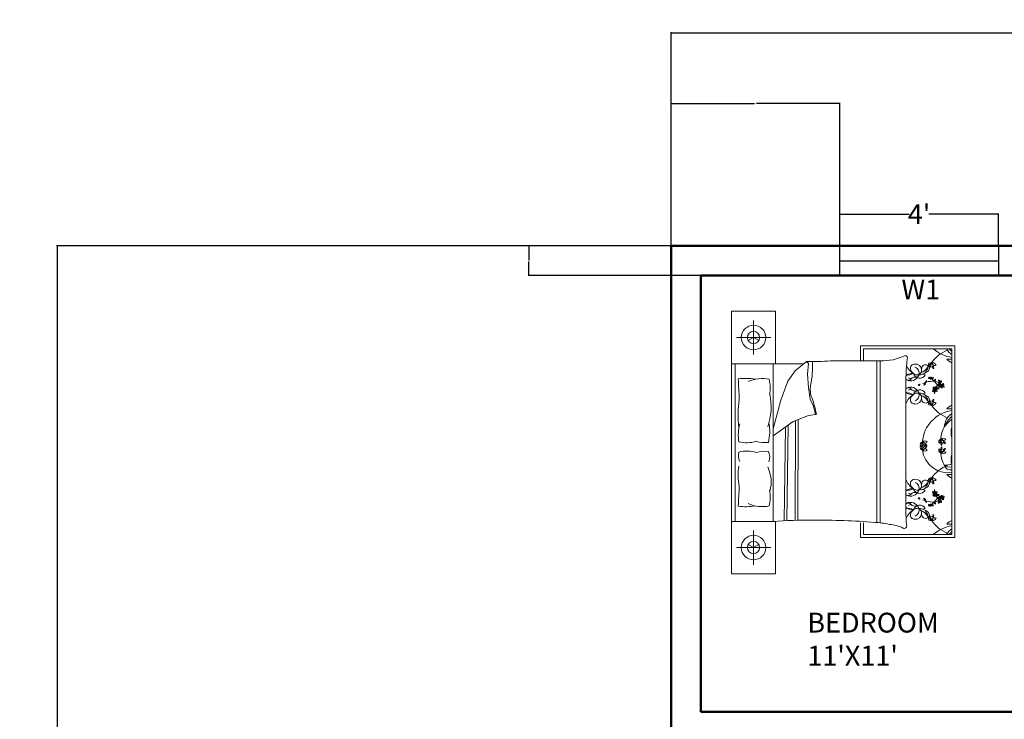
# Model space of a CAD drawing. Units: inches. Extents: x -173 to 545, y -746 to 104.
# Tile 22 of 32: x -173 to 125, y -127 to 85. Entities that reach past the tile are written whole.
import ezdxf

# ---------------------------------------------------------------- set-up
doc = ezdxf.new("R2010")
doc.units = ezdxf.units.IN
doc.header["$MEASUREMENT"] = 0
for name, color, linetype, lineweight in [('A-ANNO-DIMS', 2, 'Continuous', 18), ('A-ANNO-TEXT', 7, 'Continuous', 18), ('A-AREA-IDEN', 7, 'Continuous', 18), ('A-FURN', 8, 'Continuous', 18), ('A-GLAZ', 3, 'Continuous', 25), ('A-WALL', 7, 'Continuous', 50)]:
    doc.layers.add(name, color=color, linetype=linetype, lineweight=lineweight)
doc.styles.get("Standard").update_dxf_attribs({"font": 'arial.ttf'})
doc.dimstyles.get("Standard").update_dxf_attribs({"dimtxt": 0.18, "dimasz": 0.18, "dimexe": 0.18, "dimexo": 0.0625, "dimgap": 0.09, "dimtad": 0, "dimtih": 1, "dimtoh": 1, "dimdec": 0, "dimzin": 0, "dimdsep": 46, "dimlunit": 3, "dimtxsty": 'Standard', "dimcen": 0.09, "dimadec": 0, "dimazin": 0, "dimtfac": 1, "dimtdec": 0, "dimtofl": 0, "dimtmove": 0, "dimatfit": 3, "dimfxl": 1, "dimtolj": 1, "dimtzin": 0, "dimarcsym": 0})

# ---------------------------------------------------------------- blocks, each defined once
blk = doc.blocks.new('*D9')
at = {"layer": 'A-ANNO-DIMS', "color": 0, "lineweight": -2, "transparency": 16777216}
for p, q in [((75.3, 16.7), (75.3, 26.42)), ((75.48, 26.24), (96.33, 26.24)), ((123.12, 26.24), (102.27, 26.24)), ((123.3, 16.7), (123.3, 26.42))]:
    blk.add_line(p, q, dxfattribs=at)
at = {"layer": 'A-ANNO-DIMS', "color": 0, "transparency": 16777216}
for points in [[(75.48, 26.27), (75.48, 26.21), (75.3, 26.24)], [(123.12, 26.27), (123.12, 26.21), (123.3, 26.24)]]:
    blk.add_solid(points, dxfattribs=at)
at = {"layer": 'Defpoints', "color": 0, "transparency": 16777216}
for p in [(123.3, 26.24), (75.3, 16.64), (123.3, 16.64)]:
    blk.add_point(p, dxfattribs=at)
at = {"layer": 'A-ANNO-DIMS', "color": 0, "transparency": 16777216, "insert": (99.3, 26.24), "char_height": 6, "attachment_point": 5}
blk.add_mtext("\\A1;4'", dxfattribs=at)
blk = doc.blocks.new('*D23')
at = {"layer": 'A-ANNO-DIMS', "color": 0, "lineweight": -2, "transparency": 16777216}
for p, q in [((24.3, 16.7), (24.3, 81.33)), ((24.48, 81.15), (250.33, 81.15)), ((501.62, 81.15), (275.78, 81.15)), ((501.8, 16.7), (501.8, 81.33))]:
    blk.add_line(p, q, dxfattribs=at)
at = {"layer": 'A-ANNO-DIMS', "color": 0, "transparency": 16777216}
for points in [[(24.48, 81.18), (24.48, 81.12), (24.3, 81.15)], [(501.62, 81.18), (501.62, 81.12), (501.8, 81.15)]]:
    blk.add_solid(points, dxfattribs=at)
at = {"layer": 'Defpoints', "color": 0, "transparency": 16777216}
for p in [(501.8, 81.15), (24.3, 16.64), (501.8, 16.64)]:
    blk.add_point(p, dxfattribs=at)
at = {"layer": 'A-ANNO-DIMS', "color": 0, "transparency": 16777216, "insert": (263.05, 81.15), "char_height": 6, "attachment_point": 5}
blk.add_mtext('\\A1;39\'-10"', dxfattribs=at)
blk = doc.blocks.new('*D24')
at = {"layer": 'A-ANNO-DIMS', "color": 0, "lineweight": -2, "transparency": 16777216}
for p, q in [((24.24, 16.64), (-161.72, 16.64)), ((-161.54, 16.46), (-161.54, -337.21)), ((-161.54, -697.18), (-161.54, -343.52)), ((24.24, -697.36), (-161.72, -697.36))]:
    blk.add_line(p, q, dxfattribs=at)
at = {"layer": 'A-ANNO-DIMS', "color": 0, "transparency": 16777216}
for points in [[(-161.57, 16.46), (-161.51, 16.46), (-161.54, 16.64)], [(-161.57, -697.18), (-161.51, -697.18), (-161.54, -697.36)]]:
    blk.add_solid(points, dxfattribs=at)
at = {"layer": 'Defpoints', "color": 0, "transparency": 16777216}
for p in [(24.3, 16.64), (-161.54, -697.36), (24.3, -697.36)]:
    blk.add_point(p, dxfattribs=at)
at = {"layer": 'A-ANNO-DIMS', "color": 0, "transparency": 16777216, "insert": (-161.54, -340.36), "char_height": 6, "attachment_point": 5}
blk.add_mtext('\\A1;59\'-6"', dxfattribs=at)
blk = doc.blocks.new('BED-SUITE-COMPACT')
for p, q in [((0, 79.47), (0, 0)), ((6.62, 66.33), (6.62, 76.71)), ((11.81, 71.52), (1.43, 71.52)), ((38.96, 68.98), (38.96, 64.48)), ((67.58, 68.98), (38.96, 68.98)), ((67.58, 11.04), (67.58, 68.98)), ((39.88, 64.49), (39.88, 68.06)), ((39.88, 68.06), (66.66, 68.06)), ((66.66, 68.06), (66.66, 11.96)), ((0, 63.58), (21.81, 63.58)), ((1.02, 15.89), (1.02, 63.58)), ((12.56, 63.58), (12.56, 15.89)), ((22.64, 64.29), (19.26, 61.39)), ((23.29, 63.64), (22.64, 64.29)), ((22.96, 60.42), (23.29, 63.64)), ((43.91, 15.53), (43.91, 64.49)), ((44.9, 15.46), (44.9, 64.49)), ((19.26, 61.39), (17.01, 58.33)), ((23.29, 56.4), (22.96, 60.42)), ((58.61, 60.23), (57.71, 60.4)), ((17.01, 58.33), (14.92, 52.54)), ((23.77, 52.86), (23.29, 56.4)), ((52.71, 23.6), (52.71, 55.87)), ((58.61, 54.67), (57.71, 54.5)), ((14.92, 52.54), (12.56, 43.87)), ((24.73, 50.77), (23.77, 52.86)), ((25.38, 48.19), (24.73, 50.77)), ((18.62, 46.1), (23.29, 47.87)), ((23.29, 47.87), (25.38, 48.19)), ((12.56, 41.74), (18.62, 46.1)), ((16.68, 16.14), (17.08, 44.99)), ((19.18, 16.18), (19.3, 46.36)), ((19.99, 16.17), (20.12, 46.67)), ((15.86, 16.11), (16.26, 44.4)), ((58.61, 25.35), (57.71, 25.53)), ((58.61, 19.8), (57.71, 19.62)), ((38.96, 15.45), (38.96, 11.04)), ((39.88, 11.96), (39.88, 15.47)), ((6.62, 13.14), (6.62, 2.75)), ((66.66, 11.96), (39.88, 11.96)), ((38.96, 11.04), (67.58, 11.04)), ((11.81, 7.95), (1.43, 7.95))]:
    blk.add_line(p, q)
for points in [[(13.24, 63.58), (13.24, 79.47), (0, 79.47)], [(6.62, 71.52), (5.02, 70.6)], [(6.62, 71.52), (8.23, 70.6)], [(0, 15.89), (13.24, 15.89), (13.24, 0), (0, 0)], [(6.62, 7.95), (5.02, 8.87)], [(6.62, 7.95), (8.23, 8.87)]]:
    blk.add_lwpolyline(points)
for points in [[(29.92, 64.45, -0.001242), (45, 64.49, 0.127202), (52.51, 66.08)], [(1.98, 59.01, -0.074897), (7.17, 58.91, 0.472817)], [(7.46, 40.11, -0.14099), (2.17, 39.95, -0.235245)], [(7.46, 36.71, 0.14099), (2.17, 36.87, 0.235245)], [(1.98, 20.46, 0.074897), (7.17, 20.55, -0.472817)], [(43.29, 15.55, -0.056112), (47.66, 14.98, -0.095341), (51.87, 13.86)]]:
    blk.add_lwpolyline(points, format="xyb")
for centre, radius in [((6.62, 71.52), 3.71), ((6.62, 71.52), 1.85), ((63.62, 56.96), 0.202), ((61.49, 55.64), 0.202), ((61.49, 24.39), 0.202), ((63.62, 23.06), 0.202), ((6.62, 7.95), 3.71), ((6.62, 7.95), 1.85)]:
    blk.add_circle(centre, radius)
for centre, radius, start, end in [((52.46, 65.35), 0.733, 332.6588, 86.02), ((69.09, 58.03), 10.38, 111.4092, 145.6135), ((68.06, 75.78), 10.38, 228.1144, 262.255), ((69.45, 70.58), 5.06, 209.8884, 236.5383), ((70.39, 72.4), 6.3, 223.5186, 233.6964), ((24.62, 137.15), 72.89, 268.447, 274.1706), ((-5.5, 62.93), 29.99, 348.6608, 2.5481), ((135.43, 56.82), 82.73, 174.3113, 180.6567), ((58.31, 65.66), 6.01, 206.7003, 236.3329), ((55.42, 62.16), 1.34, 88.9462, 185.5144), ((55.61, 61.61), 1.9, 7.1143, 95.0551), ((54.89, 60.86), 1.84, 338.5779, 68.4181), ((58.67, 62.05), 1.19, 19.1312, 189.736), ((59.96, 62.29), 0.731, 126.7319, 206.0245), ((60.32, 63.06), 0.86, 76.272, 177.0484), ((59.01, 64.81), 1.77, 284.7031, 328.6173), ((61.48, 62.56), 1.64, 125.7657, 194.5347), ((53.44, 65.47), 7.26, 332.8176, 347.4827), ((60.77, 62.77), 1.15, 20.9613, 102.2885), ((61.39, 63.92), 0.867, 181.7131, 301.5367), ((58.55, 62.16), 2.62, 2.0648, 41.1598), ((60.13, 63.14), 0.849, 316.2238, 62.3173), ((60.66, 62.63), 0.112, 20.2817, 316.2238), ((68.28, 67.75), 4.22, 221.0454, 247.4453), ((66.01, 79.3), 14.36, 266.3481, 272.5919), ((53.59, 59.38), 0.957, 127.675, 149.9707), ((53.3, 63.46), 3.29, 260.8446, 301.1782), ((54.15, 60.91), 2.53, 240.8249, 340.7178), ((54.73, 57.6), 3.06, 85.2696, 124.215), ((56.41, 62.57), 2.39, 193.079, 274.7067), ((56.89, 61.21), 1.98, 196.8663, 330.0915), ((56.06, 59.96), 0.493, 254.8529, 12.6959), ((54.73, 57.6), 3.06, 53.6555, 57.2989), ((55.19, 61.94), 2.31, 305.9599, 357.6409), ((56.35, 64.45), 4.26, 273.4924, 303.7117), ((56.04, 64.41), 3.75, 288.2955, 328.7386), ((58.31, 62.33), 1.49, 285.6955, 4.031), ((60.29, 60.73), 1.59, 128.4175, 173.8338), ((60.98, 62.27), 0.0626, 52.0591, 168.5166), ((61.04, 62.25), 0.129, 168.5166, 2.0648), ((-754.3, 15.21), 757.55, 2.85022, 3.31479), ((9.26, 48.89), 10.24, 78.2417, 114.8684), ((1.05, 56.18), 10.65, 348.9631, 14.8961), ((30.25, 55.76), 6.47, 168.6608, 203.7384), ((53.59, 59.38), 0.957, 206.442, 225.5483), ((53.4, 59.78), 1.19, 246.1646, 318.4347), ((54.61, 61.29), 2.28, 240.0851, 262.564), ((55.51, 57.91), 1.63, 74.8529, 138.4347), ((56.72, 57.24), 0.249, 169.5864, 349.5616), ((56.81, 57.22), 0.153, 349.5616, 167.2949), ((60.81, 51.71), 6.58, 110.1059, 116.9968), ((58.6, 57.14), 0.417, 129.5056, 182.6421), ((57.41, 58.1), 1.26, 308.4388, 328.836), ((57.19, 59.13), 2.24, 296.5064, 305.3102), ((57.17, 57.97), 1.28, 336.3901, 344.4871), ((58.56, 57.65), 0.162, 83.9457, 185.6216), ((57.91, 57.8), 0.666, 328.836, 0.8141), ((58.25, 57.6), 0.381, 306.5232, 32.4668), ((58.71, 57.9), 0.162, 112.5583, 214.2343), ((58.6, 58.19), 0.381, 265.7131, 351.6568), ((58.27, 58.4), 0.666, 297.3659, 329.344), ((57.77, 58.97), 1.28, 313.6929, 321.7899), ((59.18, 58.1), 0.417, 115.5379, 168.6744), ((57.76, 58.7), 1.26, 329.344, 349.7412), ((60.81, 51.71), 6.58, 86.1723, 106.4158), ((56.76, 58.41), 2.24, 352.8698, 1.6736), ((59.73, 59.22), 0.156, 125.0752, 284.7644), ((59.97, 59.28), 0.338, 127.3642, 168.4363), ((59.7, 59.55), 0.487, 277.4968, 341.2737), ((60.09, 59.32), 0.193, 88.1325, 178.8919), ((60.48, 59.12), 0.418, 136.3462, 189.6513), ((60.24, 59.08), 0.174, 189.6513, 312.3208), ((60.28, 59.56), 0.202, 183.2768, 356.7232), ((60.91, 59.2), 0.663, 164.2829, 186.9148), ((60.13, 59.19), 0.331, 312.3208, 40.2111), ((60.83, 59.57), 0.47, 201.6382, 274.947), ((60.21, 58.92), 0.614, 42.3896, 66.5724), ((66.41, 63.79), 7.55, 217.9541, 226.8459), ((60.66, 59.28), 0.334, 10.9597, 52.2379), ((60.86, 59.25), 0.155, 274.947, 37.5263), ((61.18, 57.19), 0.923, 253.6301, 325.4631), ((61.38, 58.37), 0.162, 112.5583, 214.2343), ((61.28, 58.66), 0.381, 265.7131, 351.6568), ((60.94, 58.87), 0.666, 297.3659, 329.344), ((60.98, 54.99), 3.3, 60.7959, 85.244), ((53.95, 50.24), 10.86, 37.8256, 47.7588), ((60.44, 59.45), 1.28, 313.6929, 321.7899), ((61.39, 56.69), 0.561, 273.8774, 357.1501), ((61.85, 58.57), 0.417, 115.5379, 168.6744), ((60.44, 59.17), 1.26, 329.344, 349.7412), ((61.61, 57.09), 0.543, 262.0748, 308.2393), ((59.43, 58.88), 2.24, 352.8698, 1.6736), ((62.39, 56.98), 0.543, 215.1128, 261.2773), ((62.82, 56.95), 0.923, 197.889, 269.722), ((65.36, 54.65), 3.96, 130.182, 149.456), ((62.58, 58.43), 0.226, 33.0979, 123.1364), ((57.61, 55.25), 5.91, 31.1156, 34.8118), ((62.26, 58.05), 0.612, 2.3172, 70.5201), ((63.18, 56.91), 0.653, 139.3812, 199.9959), ((61.96, 57.38), 0.923, 310.9365, 22.7695), ((62.39, 57.33), 0.67, 285.6484, 332.2957), ((62.76, 57.89), 0.177, 135.7354, 318.1297), ((62.47, 58.18), 0.234, 315.7354, 31.1156), ((62.27, 57.69), 0.543, 319.3812, 5.5456), ((62.89, 57.9), 0.177, 68.2452, 250.6395), ((62.49, 58.11), 0.527, 352.6008, 57.1845), ((64.37, 54.58), 3.52, 111.7087, 116.2181), ((60.98, 54.99), 3.3, 47.5083, 55.9967), ((62.99, 58.23), 0.527, 252.8042, 349.6943), ((62.49, 57.29), 0.561, 331.1838, 51.6792), ((63.06, 56.62), 0.156, 125.0752, 284.7644), ((63.05, 58.28), 0.234, 248.2452, 323.6254), ((63.31, 56.68), 0.338, 93.635, 168.4363), ((63.26, 57.21), 0.198, 138.2946, 276.2474), ((62.84, 58.42), 0.612, 291.7087, 3.0299), ((63.04, 56.95), 0.487, 277.4968, 341.2737), ((63.34, 57.18), 0.276, 358.5719, 143.8954), ((58.47, 61.64), 5.91, 323.6254, 327.3216), ((63.43, 56.72), 0.193, 88.1325, 178.8919), ((63.5, 57.4), 0.279, 208.8493, 269.9355), ((63.26, 57.33), 0.318, 274.2123, 318.1587), ((63.82, 56.52), 0.418, 136.3462, 189.6513), ((63.32, 58.27), 0.226, 325.6077, 55.6462), ((64.25, 56.6), 0.663, 164.2829, 186.9148), ((64.23, 57.01), 0.638, 121.9501, 165.2442), ((63.47, 56.59), 0.331, 312.3208, 40.2111), ((64.17, 56.97), 0.47, 201.6382, 274.947), ((63.79, 57.26), 0.134, 262.868, 7.094), ((63.55, 56.32), 0.614, 42.3896, 66.5724), ((63.77, 57.37), 0.399, 278.5614, 22.5914), ((63.99, 56.68), 0.334, 10.9597, 118.7804), ((64, 57.39), 0.201, 44.3732, 121.9501), ((64.2, 56.65), 0.155, 274.947, 37.5263), ((-6.52, 50.57), 18.47, 340.7385, 11.9603), ((53.59, 55.52), 0.957, 134.4517, 156.771), ((53.59, 55.52), 0.957, 203.2856, 232.325), ((53.3, 51.45), 3.29, 58.8218, 100.2867), ((58.31, 49.24), 6.01, 123.6671, 158.5059), ((54.15, 54), 2.53, 19.2822, 119.1751), ((53.4, 55.12), 1.19, 41.5653, 113.8354), ((54.73, 57.3), 3.06, 235.785, 274.7304), ((54.61, 53.61), 2.28, 97.436, 119.9149), ((56.41, 52.33), 2.39, 85.2933, 166.921), ((55.51, 56.99), 1.63, 221.5653, 285.1471), ((56.89, 53.69), 1.98, 29.9085, 163.1337), ((54.89, 54.04), 1.84, 291.5819, 21.4221), ((56.06, 54.94), 0.493, 347.3041, 105.1471), ((54.73, 57.3), 3.06, 302.7011, 306.3445), ((55.19, 52.96), 2.31, 2.3591, 54.0401), ((56.35, 50.46), 4.26, 56.2883, 86.5076), ((56.04, 50.49), 3.75, 31.2614, 71.7045), ((60.29, 54.17), 1.59, 186.1662, 231.5825), ((58.31, 52.57), 1.49, 355.969, 74.3045), ((60.93, 55.3), 0.156, 125.0752, 284.7644), ((61.17, 55.36), 0.338, 93.635, 168.4363), ((61.44, 55.91), 0.653, 82.0748, 142.6895), ((61.37, 56.8), 0.67, 228.342, 274.9894), ((61.13, 55.89), 0.198, 138.2946, 276.2474), ((60.91, 55.63), 0.487, 277.4968, 341.2737), ((61.2, 55.86), 0.276, 358.5719, 143.8954), ((61.29, 55.4), 0.193, 88.1325, 178.8919), ((61.36, 56.08), 0.279, 208.8493, 269.9355), ((61.13, 56.01), 0.318, 274.2123, 318.1587), ((61.68, 55.2), 0.418, 136.3462, 189.6513), ((61.44, 55.15), 0.174, 189.6513, 312.3208), ((65.36, 54.65), 3.96, 175.2415, 182.8929), ((62.12, 55.27), 0.663, 164.2829, 186.9148), ((62.1, 55.69), 0.638, 121.9501, 165.2442), ((61.34, 55.27), 0.331, 312.3208, 40.2111), ((62.04, 55.64), 0.47, 201.6382, 274.947), ((61.66, 55.94), 0.134, 262.868, 7.094), ((61.41, 55), 0.614, 42.3896, 66.5724), ((61.64, 56.05), 0.399, 278.5614, 22.5914), ((61.86, 55.36), 0.334, 10.9597, 118.7804), ((65.36, 54.65), 3.96, 156.1523, 156.9499), ((61.87, 56.06), 0.201, 44.3732, 121.9501), ((62.48, 56.53), 0.561, 181.4625, 249.4747), ((62.06, 55.33), 0.155, 274.947, 37.5263), ((62.53, 56.63), 0.67, 248.3627, 295.0101), ((62.21, 55.79), 0.653, 20.6625, 81.2773), ((63.58, 56.48), 0.174, 189.6513, 312.3208), ((30.74, 48.12), 28.82, 170.503, 187.7804), ((-4.65, 42.67), 30.82, 10.6617, 19.8806), ((55.42, 52.74), 1.34, 174.4856, 271.0538), ((55.61, 53.29), 1.9, 264.9449, 352.8857), ((58.67, 52.86), 1.19, 170.264, 340.8688), ((59.96, 52.61), 0.731, 153.9755, 233.2681), ((60.32, 51.85), 0.86, 182.9516, 283.728), ((59.01, 50.09), 1.77, 31.3827, 75.2969), ((61.48, 52.34), 1.64, 165.4653, 234.2343), ((53.44, 49.44), 7.26, 12.5173, 27.1824), ((58.55, 52.74), 2.62, 318.8402, 357.9352), ((60.13, 51.76), 0.849, 297.6827, 43.7762), ((61.39, 50.98), 0.867, 58.4633, 178.2869), ((60.77, 52.13), 1.15, 257.7115, 339.0387), ((69.09, 56.87), 10.38, 214.3865, 248.5908), ((60.62, 52.26), 0.0677, 43.7729, 339.7333), ((61.04, 52.65), 0.129, 357.9352, 191.4834), ((60.98, 52.63), 0.0626, 191.4834, 307.9409), ((68.28, 47.15), 4.22, 112.5547, 138.9546), ((25.44, 48.37), 0.192, 250.2464, 1.1377), ((68.06, 39.12), 10.38, 97.745, 175.5377), ((69.45, 44.32), 5.06, 123.4617, 178.728), ((66.01, 35.6), 14.36, 87.4081, 93.6519), ((16.17, 42.03), 14.16, 166.04, 188.4751), ((-2.49, 43.09), 14.01, 346.3762, 10.1383), ((70.39, 42.5), 6.3, 126.3036, 162.1496), ((72.17, 39.19), 9.37, 125.947, 145.9877), ((73.62, 39.91), 10.38, 152.5854, 175.5377), ((72.12, 42.81), 5.71, 162.9798, 196.4569), ((10.12, 49.47), 9.74, 254.1707, 275.9871), ((57.95, 39.1), 0.86, 106.1963, 206.9726), ((55.94, 39.97), 1.77, 314.6273, 358.5415), ((59.21, 39.25), 1.64, 155.6899, 224.4589), ((59.21, 38.13), 1.64, 135.5411, 204.3101), ((58.49, 39.07), 1.15, 50.8855, 132.2127), ((58.45, 40.38), 0.867, 211.6373, 331.4609), ((50.79, 37.75), 7.26, 2.7418, 17.407), ((57.75, 39.08), 0.849, 346.148, 92.2415), ((56.86, 37.44), 2.62, 31.989, 71.0841), ((50.79, 39.62), 7.26, 342.593, 357.2582), ((58.46, 38.9), 0.112, 50.0755, 346.148), ((58.98, 38.76), 0.129, 198.4408, 31.989), ((58.92, 38.74), 0.0626, 81.9833, 198.4408), ((58.98, 38.61), 0.129, 328.011, 161.5592), ((63.51, 39.89), 0.86, 106.1963, 206.9726), ((61.5, 40.76), 1.77, 314.6273, 358.5415), ((64.77, 40.04), 1.64, 155.6899, 224.4589), ((64.05, 39.87), 1.15, 50.8855, 132.2127), ((64.01, 41.17), 0.867, 211.6373, 331.4609), ((62.42, 38.24), 2.62, 31.989, 71.0841), ((56.35, 38.55), 7.26, 2.7418, 17.407), ((63.31, 39.87), 0.849, 346.148, 92.2415), ((64.02, 39.69), 0.112, 50.0755, 346.148), ((64.48, 39.54), 0.0626, 81.9833, 198.4408), ((64.54, 39.56), 0.129, 198.4408, 31.989), ((75.06, 40.55), 8.44, 174.3643, 175.6213), ((80.84, 36.11), 15.08, 160.0972, 160.2783), ((5.94, 35.78), 3.93, 163.8974, 206.6563), ((10.12, 27.35), 9.74, 84.0129, 105.8293), ((7.31, 35.25), 4.21, 341.4593, 24.9817), ((57.95, 38.28), 0.86, 153.0274, 253.8037), ((55.94, 37.41), 1.77, 1.4585, 45.3727), ((56.86, 39.93), 2.62, 288.9159, 328.011), ((57.75, 38.3), 0.849, 267.7585, 13.852), ((58.45, 37), 0.867, 28.5391, 148.3627), ((58.49, 38.3), 1.15, 227.7873, 309.1145), ((65.66, 38.59), 8.03, 188.1803, 277.1364), ((58.42, 38.49), 0.0677, 13.9791, 309.8091), ((58.92, 38.63), 0.0626, 161.5592, 278.0167), ((63.51, 37.48), 0.86, 153.0274, 253.8037), ((61.5, 36.61), 1.77, 1.4585, 45.3727), ((64.77, 37.33), 1.64, 135.5411, 204.3101), ((56.35, 38.83), 7.26, 342.593, 357.2582), ((62.42, 39.14), 2.62, 288.9159, 328.011), ((63.31, 37.5), 0.849, 267.7585, 13.852), ((64.01, 36.2), 0.867, 28.5391, 148.3627), ((64.05, 37.51), 1.15, 227.7873, 309.1145), ((73.62, 37.46), 10.38, 184.4623, 207.4146), ((63.98, 37.69), 0.0677, 13.9791, 309.8091), ((64.48, 37.84), 0.0626, 161.5592, 278.0167), ((64.54, 37.82), 0.129, 328.011, 161.5592), ((72.12, 34.56), 5.71, 163.5431, 197.0202), ((75.06, 36.82), 8.44, 184.3787, 185.6357), ((80.84, 41.27), 15.08, 199.7217, 199.9028), ((69.09, 23.15), 10.38, 111.4092, 145.6135), ((64.93, 37.55), 4.65, 263.3805, 291.883), ((66.22, 33.29), 1.86, 190.9261, 283.6102), ((65.97, 34.69), 2.36, 228.0951, 287.1391), ((15.89, 29.89), 13.97, 168.8159, 193.6573), ((1.84, 27.89), 10.12, 343.8254, 26.1239), ((66.01, 44.43), 14.36, 266.3481, 272.5919), ((68.28, 32.87), 4.22, 221.0454, 247.4453), ((58.31, 30.78), 6.01, 201.4941, 236.3329), ((55.42, 27.28), 1.34, 88.9462, 185.5144), ((56.41, 27.69), 2.39, 193.079, 274.7067), ((55.61, 26.73), 1.9, 7.1143, 95.0551), ((54.89, 25.98), 1.84, 338.5779, 68.4181), ((55.19, 27.06), 2.31, 305.9599, 357.6409), ((56.04, 29.53), 3.75, 288.2955, 328.7386), ((58.67, 27.17), 1.19, 19.1312, 189.736), ((58.31, 27.45), 1.49, 285.6955, 4.031), ((60.29, 25.85), 1.59, 128.4175, 173.8338), ((59.96, 27.41), 0.731, 126.7319, 206.0245), ((60.32, 28.18), 0.86, 76.272, 177.0484), ((59.01, 29.94), 1.77, 284.7031, 328.6173), ((61.48, 27.68), 1.64, 125.7657, 194.5347), ((53.44, 30.59), 7.26, 332.8176, 347.4827), ((60.77, 27.89), 1.15, 20.9613, 102.2885), ((60.13, 28.26), 0.849, 316.2238, 62.3173), ((58.55, 27.29), 2.62, 2.0648, 41.1598), ((61.39, 29.04), 0.867, 181.7131, 301.5367), ((60.66, 27.75), 0.112, 20.2817, 316.2238), ((60.98, 27.39), 0.0626, 52.0591, 168.5166), ((61.04, 27.38), 0.129, 168.5166, 2.0648), ((-754.3, 64.26), 757.55, 356.68521, 357.14978), ((1.05, 23.29), 10.65, 345.1039, 11.0369), ((53.3, 28.58), 3.29, 259.7133, 301.1782), ((53.59, 24.5), 0.957, 127.675, 156.7144), ((53.59, 24.5), 0.957, 203.2856, 225.5483), ((54.15, 26.03), 2.53, 240.8249, 340.7178), ((53.4, 24.9), 1.19, 246.1646, 318.4347), ((54.73, 22.72), 3.06, 85.2696, 124.215), ((54.61, 26.41), 2.28, 240.0851, 262.564), ((55.51, 23.04), 1.63, 74.8529, 138.4347), ((56.89, 26.33), 1.98, 196.8663, 330.0915), ((56.06, 25.08), 0.493, 254.8529, 12.6959), ((54.73, 22.72), 3.06, 53.6555, 57.2989), ((56.35, 29.57), 4.26, 273.4924, 303.7117), ((60.93, 24.73), 0.156, 75.2356, 234.9248), ((61.17, 24.67), 0.338, 191.5637, 266.365), ((61.37, 23.22), 0.67, 85.0106, 131.658), ((61.13, 24.13), 0.198, 83.7526, 221.7054), ((60.91, 24.4), 0.487, 18.7263, 82.5032), ((61.2, 24.16), 0.276, 216.1046, 1.4281), ((61.29, 24.62), 0.193, 181.1081, 271.8675), ((61.36, 23.95), 0.279, 90.0645, 151.1507), ((61.13, 24.01), 0.318, 41.8413, 85.7877), ((61.68, 24.83), 0.418, 170.3487, 223.6538), ((61.44, 24.87), 0.174, 47.6792, 170.3487), ((65.36, 25.37), 3.96, 177.1071, 184.7585), ((61.39, 23.33), 0.561, 2.8499, 86.1226), ((62.12, 24.75), 0.663, 173.0852, 195.7171), ((62.1, 24.33), 0.638, 194.7558, 238.0499), ((61.34, 24.75), 0.331, 319.7889, 47.6792), ((62.04, 24.38), 0.47, 85.053, 158.3618), ((61.66, 24.09), 0.134, 352.906, 97.132), ((61.41, 25.02), 0.614, 293.4276, 317.6104), ((61.86, 24.66), 0.334, 241.2196, 349.0403), ((61.64, 23.97), 0.399, 337.4086, 81.4386), ((62.48, 23.49), 0.561, 110.5253, 178.5375), ((62.82, 23.08), 0.923, 90.278, 162.111), ((62.06, 24.69), 0.155, 322.4737, 85.053), ((62.53, 23.39), 0.67, 64.9899, 111.6373), ((62.21, 24.23), 0.653, 278.7227, 339.3375), ((9.26, 30.58), 10.24, 245.1316, 281.7583), ((130, 21.17), 77.33, 178.1965, 184.7598), ((53.59, 20.64), 0.957, 134.4517, 163.3657), ((54.15, 19.12), 2.53, 19.2822, 119.1751), ((53.4, 20.24), 1.19, 41.5653, 113.8354), ((54.61, 18.73), 2.28, 97.436, 119.9149), ((55.51, 22.11), 1.63, 221.5653, 285.1471), ((56.72, 22.78), 0.249, 10.4384, 190.4136), ((56.81, 22.8), 0.153, 192.7051, 10.4384), ((60.81, 28.31), 6.58, 243.0032, 249.8941), ((57.41, 21.92), 1.26, 31.164, 51.5612), ((58.6, 22.88), 0.417, 177.3579, 230.4944), ((57.19, 20.9), 2.24, 54.6898, 63.4936), ((57.17, 22.05), 1.28, 15.5129, 23.6099), ((58.56, 22.38), 0.162, 174.3784, 276.0543), ((58.25, 22.42), 0.381, 327.5332, 53.4768), ((57.91, 22.22), 0.666, 359.1859, 31.164), ((58.71, 22.12), 0.162, 145.7657, 247.4417), ((58.6, 21.83), 0.381, 8.3432, 94.2869), ((58.27, 21.62), 0.666, 30.656, 62.6341), ((57.77, 21.05), 1.28, 38.2101, 46.3071), ((59.18, 21.92), 0.417, 191.3256, 244.4621), ((57.76, 21.32), 1.26, 10.2588, 30.656), ((60.81, 28.31), 6.58, 253.5842, 273.8277), ((56.76, 21.61), 2.24, 358.3264, 7.1302), ((59.73, 20.8), 0.156, 75.2356, 234.9248), ((59.7, 20.47), 0.487, 18.7263, 82.5032), ((60.48, 20.9), 0.418, 170.3487, 223.6538), ((60.24, 20.95), 0.174, 47.6792, 170.3487), ((60.91, 20.83), 0.663, 173.0852, 195.7171), ((60.13, 20.83), 0.331, 319.7889, 47.6792), ((60.83, 20.46), 0.47, 85.053, 158.3618), ((66.41, 16.24), 7.55, 133.1541, 142.0459), ((60.86, 20.77), 0.155, 322.4737, 85.053), ((61.18, 22.84), 0.923, 34.5369, 106.3699), ((61.44, 24.12), 0.653, 217.3105, 277.9252), ((61.38, 21.65), 0.162, 145.7657, 247.4417), ((53.95, 29.78), 10.86, 312.2412, 322.1744), ((60.98, 25.03), 3.3, 274.756, 299.2041), ((61.28, 21.36), 0.381, 8.3432, 94.2869), ((60.94, 21.15), 0.666, 30.656, 62.6341), ((60.44, 20.58), 1.28, 38.2101, 46.3071), ((61.85, 21.45), 0.417, 191.3256, 244.4621), ((60.44, 20.85), 1.26, 10.2588, 30.656), ((61.61, 22.93), 0.543, 51.7607, 97.9252), ((59.43, 21.14), 2.24, 358.3264, 7.1302), ((65.36, 25.37), 3.96, 203.0501, 203.8477), ((61.87, 23.96), 0.201, 238.0499, 315.6268), ((62.39, 23.05), 0.543, 98.7227, 144.8872), ((65.36, 25.37), 3.96, 210.544, 229.818), ((62.26, 21.98), 0.612, 289.4799, 357.6828), ((57.61, 24.78), 5.91, 325.1882, 328.8844), ((62.58, 21.59), 0.226, 236.8636, 326.9021), ((63.18, 23.12), 0.653, 160.0041, 220.6188), ((61.96, 22.64), 0.923, 337.2305, 49.0635), ((62.39, 22.69), 0.67, 27.7043, 74.3516), ((62.76, 22.13), 0.177, 41.8703, 224.2646), ((62.47, 21.84), 0.234, 328.8844, 44.2646), ((62.27, 22.34), 0.543, 354.4544, 40.6188), ((62.89, 22.13), 0.177, 109.3605, 291.7548), ((62.49, 21.91), 0.527, 302.8155, 7.3992), ((64.37, 25.45), 3.52, 243.7819, 248.2913), ((60.98, 25.03), 3.3, 304.0033, 312.4917), ((62.49, 22.73), 0.561, 308.3208, 28.8162), ((62.99, 21.79), 0.527, 10.3057, 107.1958), ((63.06, 23.4), 0.156, 75.2356, 234.9248), ((63.05, 21.75), 0.234, 36.3746, 111.7548), ((63.31, 23.34), 0.338, 191.5637, 266.365), ((63.26, 22.81), 0.198, 83.7526, 221.7054), ((62.84, 21.6), 0.612, 356.9701, 68.2913), ((63.04, 23.07), 0.487, 18.7263, 82.5032), ((63.34, 22.84), 0.276, 216.1046, 1.4281), ((63.43, 23.3), 0.193, 181.1081, 271.8675), ((58.47, 18.38), 5.91, 32.6784, 36.3746), ((63.5, 22.62), 0.279, 90.0645, 151.1507), ((63.26, 22.69), 0.318, 41.8413, 85.7877), ((63.58, 23.55), 0.174, 47.6792, 170.3487), ((63.82, 23.5), 0.418, 170.3487, 223.6538), ((63.32, 21.76), 0.226, 304.3538, 34.3923), ((64.25, 23.42), 0.663, 173.0852, 195.7171), ((64.23, 23.01), 0.638, 194.7558, 238.0499), ((63.47, 23.43), 0.331, 319.7889, 47.6792), ((64.17, 23.06), 0.47, 85.053, 158.3618), ((63.79, 22.76), 0.134, 352.906, 97.132), ((63.55, 23.7), 0.614, 293.4276, 317.6104), ((63.99, 23.34), 0.334, 241.2196, 349.0403), ((63.77, 22.65), 0.399, 337.4086, 81.4386), ((64, 22.64), 0.201, 238.0499, 315.6268), ((64.2, 23.37), 0.155, 322.4737, 85.053), ((53.59, 20.64), 0.957, 197.4186, 232.325), ((53.3, 16.57), 3.29, 58.8218, 100.751), ((58.31, 14.36), 6.01, 123.6671, 156.3547), ((54.73, 22.42), 3.06, 235.785, 274.7304), ((56.41, 17.45), 2.39, 85.2933, 166.921), ((55.42, 17.86), 1.34, 174.4856, 271.0538), ((56.89, 18.81), 1.98, 29.9085, 163.1337), ((55.61, 18.41), 1.9, 264.9449, 352.8857), ((54.89, 19.16), 1.84, 291.5819, 21.4221), ((56.06, 20.06), 0.493, 347.3041, 105.1471), ((54.73, 22.42), 3.06, 302.7011, 306.3445), ((55.19, 18.08), 2.31, 2.3591, 54.0401), ((56.35, 15.58), 4.26, 56.2883, 86.5076), ((56.04, 15.61), 3.75, 31.2614, 71.7045), ((58.67, 17.98), 1.19, 170.264, 340.8688), ((58.31, 17.69), 1.49, 355.969, 74.3045), ((60.29, 19.3), 1.59, 186.1662, 231.5825), ((59.96, 17.73), 0.731, 153.9755, 233.2681), ((59.97, 20.74), 0.338, 191.5637, 232.6358), ((60.09, 20.7), 0.193, 181.1081, 271.8675), ((60.28, 20.46), 0.202, 3.2768, 176.7232), ((60.21, 21.1), 0.614, 293.4276, 317.6104), ((60.66, 20.74), 0.334, 307.7621, 349.0403), ((61.04, 17.77), 0.129, 357.9352, 191.4834), ((22.27, -126.57), 142.79, 89.0718, 93.9), ((27.46, -170.04), 186.27, 85.1265, 90.8855), ((59.01, 15.21), 1.77, 31.3827, 75.2969), ((60.32, 16.97), 0.86, 182.9516, 283.728), ((61.48, 17.46), 1.64, 165.4653, 234.2343), ((53.44, 14.56), 7.26, 12.5173, 27.1824), ((58.55, 17.86), 2.62, 318.8402, 357.9352), ((60.13, 16.88), 0.849, 297.6827, 43.7762), ((61.39, 16.11), 0.867, 58.4633, 178.2869), ((60.77, 17.26), 1.15, 257.7115, 339.0387), ((69.09, 21.99), 10.38, 214.3865, 248.5908), ((60.62, 17.38), 0.0677, 43.7729, 339.7333), ((60.98, 17.76), 0.0626, 191.4834, 307.9409), ((68.28, 12.28), 4.22, 112.5547, 138.9546), ((66.01, 0.72), 14.36, 87.4081, 93.6519), ((52.27, 14.46), 0.724, 236.1736, 23.4781), ((68.06, 4.24), 10.38, 97.745, 131.8856), ((69.45, 9.44), 5.06, 123.4617, 150.1116), ((70.39, 7.63), 6.3, 126.3036, 136.4814)]:
    blk.add_arc(centre, radius, start, end)
blk = doc.blocks.new('WINDOW-48')
for p, q in [((0, 9), (48, 9)), ((0, 0), (0, 9)), ((48, 9), (48, 0)), ((0, 4.5), (48, 4.5)), ((48, 0), (0, 0))]:
    blk.add_line(p, q)
blk = doc.blocks.new('*D78')
at = {"layer": 'A-ANNO-DIMS', "color": 0, "lineweight": -2, "transparency": 16777216}
for p, q in [((24.3, 16.7), (24.3, 59.92)), ((24.48, 59.74), (49.47, 59.74)), ((75.12, 59.74), (50.13, 59.74)), ((75.3, 16.7), (75.3, 59.92))]:
    blk.add_line(p, q, dxfattribs=at)
at = {"layer": 'A-ANNO-DIMS', "color": 0, "transparency": 16777216}
for points in [[(24.48, 59.77), (24.48, 59.71), (24.3, 59.74)], [(75.12, 59.77), (75.12, 59.71), (75.3, 59.74)]]:
    blk.add_solid(points, dxfattribs=at)
at = {"layer": 'Defpoints', "color": 0, "transparency": 16777216}
for p in [(75.3, 59.74), (24.3, 16.64), (75.3, 16.64)]:
    blk.add_point(p, dxfattribs=at)
at = {"layer": 'A-ANNO-DIMS', "color": 0, "transparency": 16777216, "insert": (49.8, 59.74), "char_height": 0.18, "attachment_point": 5}
blk.add_mtext('\\A1;4\'-3"', dxfattribs=at)
blk = doc.blocks.new('*D80')
at = {"layer": 'A-ANNO-DIMS', "color": 0, "lineweight": -2, "transparency": 16777216}
for p, q in [((75.24, 16.64), (-18.98, 16.64)), ((-18.8, 16.46), (-18.8, 12.32)), ((-18.8, 7.82), (-18.8, 11.96)), ((75.24, 7.64), (-18.98, 7.64))]:
    blk.add_line(p, q, dxfattribs=at)
at = {"layer": 'A-ANNO-DIMS', "color": 0, "transparency": 16777216}
for points in [[(-18.83, 16.46), (-18.77, 16.46), (-18.8, 16.64)], [(-18.83, 7.82), (-18.77, 7.82), (-18.8, 7.64)]]:
    blk.add_solid(points, dxfattribs=at)
at = {"layer": 'Defpoints', "color": 0, "transparency": 16777216}
for p in [(75.3, 16.64), (-18.8, 7.64), (75.3, 7.64)]:
    blk.add_point(p, dxfattribs=at)
at = {"layer": 'A-ANNO-DIMS', "color": 0, "transparency": 16777216, "insert": (-18.8, 12.14), "char_height": 0.18, "attachment_point": 5}
blk.add_mtext('\\A1;0\'-9"', dxfattribs=at)

msp = doc.modelspace()

# ---------------------------------------------------------------- linework, layer by layer
at = {"layer": 'A-WALL'}
for p, q in [((24.3, 16.64), (24.3, -697.36)), ((24.3, 16.64), (501.8, 16.64)), ((33.3, 7.64), (165.3, 7.64)), ((33.3, 7.64), (33.3, -124.36)), ((33.3, -124.36), (139.3, -124.36))]:
    msp.add_line(p, q, dxfattribs=at)

# ---------------------------------------------------------------- block references
at = {"layer": 'A-FURN'}
msp.add_blockref('BED-SUITE-COMPACT', (42.59, -82.6), dxfattribs=at)
at = {"layer": 'A-GLAZ'}
msp.add_blockref('WINDOW-48', (75.3, 7.64), dxfattribs=at)

# ---------------------------------------------------------------- texts
at = {"layer": 'A-ANNO-TEXT', "insert": (93.96, 6.46), "char_height": 6, "attachment_point": 1}
msp.add_mtext('W1', dxfattribs=at)
at = {"layer": 'A-AREA-IDEN', "insert": (65.48, -94.36), "char_height": 6, "attachment_point": 1}
msp.add_mtext("BEDROOM\\P11'X11'", dxfattribs=at)

# ---------------------------------------------------------------- dimensions: what is measured, and where the dimension line sits
at = {"layer": 'A-ANNO-DIMS'}
for base, p1, p2, override, picture, middle in [((501.80136521, 81.15311648), (24.30136521, 16.63801408), (501.80136521, 16.63801408), {"dimtxt": 6, "dimclrd": 0, "dimclre": 0, "dimclrt": 0}, '*D23', (263.05136521, 81.15311648)), ((75.3, 59.74), (24.3, 16.64), (75.3, 16.64), {"dimdec": 1, "dimlfac": 1, "dimrnd": 0, "dimzin": 1, "dimdsep": 46, "dimlunit": 4, "dimfrac": 2}, '*D78', (49.8, 59.74)), ((123.3, 26.24), (75.3, 16.64), (123.3, 16.64), {"dimtxt": 6, "dimclrd": 0, "dimclre": 0, "dimclrt": 0}, '*D9', (99.3, 26.24))]:
    dim = msp.add_linear_dim(base=base, p1=p1, p2=p2, dimstyle='Standard', override=override, dxfattribs=at)
    dim.commit()
    dim.dimension.update_dxf_attribs({"geometry": picture, "text_midpoint": middle})
for base, p1, p2, override, picture, middle in [((-161.54, -697.36), (24.3, 16.64), (24.3, -697.36), {"dimtxt": 6, "dimclrd": 0, "dimclre": 0, "dimclrt": 0}, '*D24', (-161.54, -340.36)), ((-18.8, 7.64), (75.3, 16.64), (75.3, 7.64), {"dimdec": 1, "dimlfac": 1, "dimrnd": 0, "dimzin": 1, "dimdsep": 46, "dimlunit": 4, "dimfrac": 2}, '*D80', (-18.8, 12.14))]:
    dim = msp.add_linear_dim(base=base, p1=p1, p2=p2, angle=90, dimstyle='Standard', override=override, dxfattribs=at)
    dim.commit()
    dim.dimension.update_dxf_attribs({"geometry": picture, "text_midpoint": middle})

doc.saveas('drawing.dxf')
